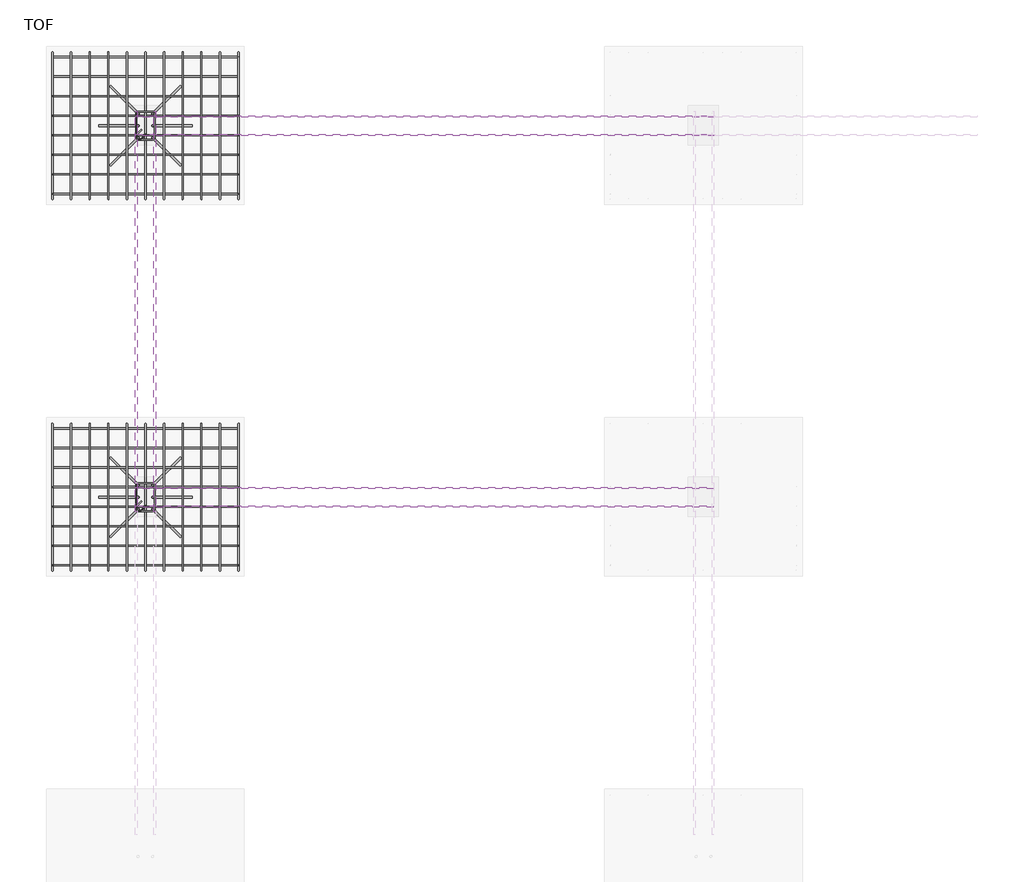
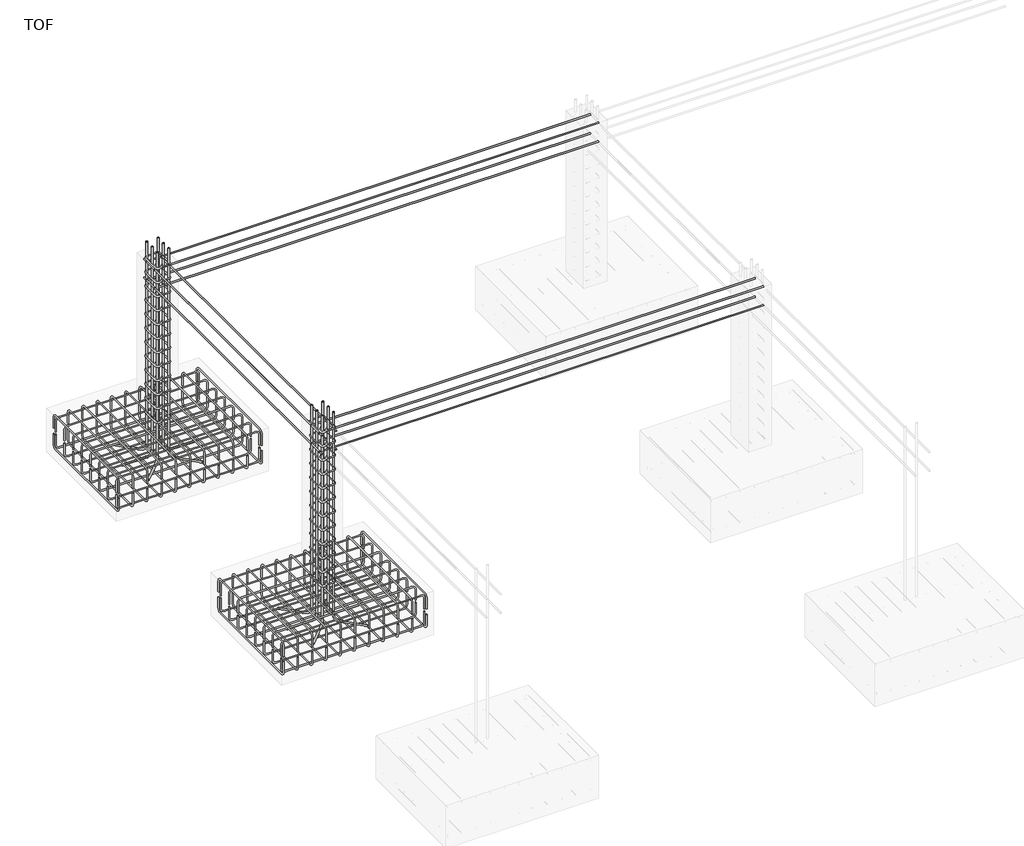
# One storey, part 3 of 10: 34 reinforcing bars.
"""IFC4 building model written with IfcOpenShell, lengths in millimetres."""

from ifc_helpers import new_model, si_unit, point, frame, origin, place, context, project, spatial, polyline, circle_curve, trimmed, segment, composite_curve, source, transform, mapped, element, save
from ifc_brep_helpers import swept_disk

model = new_model("IFC4")

# Units and contexts
model_context = context("Model", 3, world=origin())
ifc_project = project(units=[si_unit("LENGTHUNIT", "METRE", prefix="MILLI")], contexts=[model_context])

# Site, building, storey
site = spatial("IfcSite", under=ifc_project)
building = spatial("IfcBuilding", under=site)
storey = spatial("IfcBuildingStorey", under=building, Name="TOF", Elevation=-1828.8)

# Reinforcing bars
placement = place(None, origin())
reinforcing_bar_shape = source(origin(), model_context, "Body", "SolidModel", [
    swept_disk(composite_curve([segment(polyline([(-1914.7217857, -9959.6267376, -2018.8), (-1914.7217857, -9959.6267376, -1908.8)]), True, "CONTINUOUS"), segment(trimmed(circle_curve(frame((-1914.7217857, -9994.6267376, -1908.8), z_axis=(1.0, 0.0, 0.0), x_axis=(0.0, 35.0, 0.0)), 35.0), [point((-1914.7217857, -9959.6267376, -1908.8))], [point((-1914.7217857, -9994.6267376, -1873.8))], True, "CARTESIAN"), True, "CONTINUOUS"), segment(polyline([(-1914.7217857, -9994.6267376, -1873.8), (-1914.7217857, -11034.6267376, -1873.8)]), True, "CONTINUOUS"), segment(trimmed(circle_curve(frame((-1914.7217857, -11034.6267376, -1908.8), z_axis=(1.0, 0.0, 0.0), x_axis=(0.0, 0.0, 35.0)), 35.0), [point((-1914.7217857, -11034.6267376, -1873.8))], [point((-1914.7217857, -11069.6267376, -1908.8))], True, "CARTESIAN"), True, "CONTINUOUS"), segment(polyline([(-1914.7217857, -11069.6267376, -1908.8), (-1914.7217857, -11069.6267376, -2018.8)]), True, "CONTINUOUS")], self_intersect=False), 5.0),
])
element("IfcReinforcingBar", 1, at=placement, inside=storey, context=model_context, shape_type="MappedRepresentation", body=[
    mapped(reinforcing_bar_shape, transform((0.0, 0.0, 0.0), x_axis=(1.0, 0.0, 0.0), y_axis=(0.0, 1.0, 0.0), z_axis=(0.0, 0.0, 1.0))),
    mapped(reinforcing_bar_shape, transform((-141.0, 0.0, 0.0), x_axis=(1.0, 0.0, 0.0), y_axis=(0.0, 1.0, 0.0), z_axis=(0.0, 0.0, 1.0))),
    mapped(reinforcing_bar_shape, transform((-282.0, 0.0, 0.0), x_axis=(1.0, 0.0, 0.0), y_axis=(0.0, 1.0, 0.0), z_axis=(0.0, 0.0, 1.0))),
    mapped(reinforcing_bar_shape, transform((-423.0, 0.0, 0.0), x_axis=(1.0, 0.0, 0.0), y_axis=(0.0, 1.0, 0.0), z_axis=(0.0, 0.0, 1.0))),
    mapped(reinforcing_bar_shape, transform((-564.0, 0.0, 0.0), x_axis=(1.0, 0.0, 0.0), y_axis=(0.0, 1.0, 0.0), z_axis=(0.0, 0.0, 1.0))),
    mapped(reinforcing_bar_shape, transform((-705.0, 0.0, 0.0), x_axis=(1.0, 0.0, 0.0), y_axis=(0.0, 1.0, 0.0), z_axis=(0.0, 0.0, 1.0))),
    mapped(reinforcing_bar_shape, transform((-846.0, 0.0, 0.0), x_axis=(1.0, 0.0, 0.0), y_axis=(0.0, 1.0, 0.0), z_axis=(0.0, 0.0, 1.0))),
    mapped(reinforcing_bar_shape, transform((-987.0, 0.0, 0.0), x_axis=(1.0, 0.0, 0.0), y_axis=(0.0, 1.0, 0.0), z_axis=(0.0, 0.0, 1.0))),
    mapped(reinforcing_bar_shape, transform((-1128.0, 0.0, 0.0), x_axis=(1.0, 0.0, 0.0), y_axis=(0.0, 1.0, 0.0), z_axis=(0.0, 0.0, 1.0))),
    mapped(reinforcing_bar_shape, transform((-1269.0, 0.0, 0.0), x_axis=(1.0, 0.0, 0.0), y_axis=(0.0, 1.0, 0.0), z_axis=(0.0, 0.0, 1.0))),
    mapped(reinforcing_bar_shape, transform((-1410.0, 0.0, 0.0), x_axis=(1.0, 0.0, 0.0), y_axis=(0.0, 1.0, 0.0), z_axis=(0.0, 0.0, 1.0))),
])
reinforcing_bar_2_shape = source(origin(), model_context, "Body", "SolidModel", [
    swept_disk(composite_curve([segment(polyline([(-1914.7217857, -11069.6267376, -2077.5233378), (-1914.7217857, -11069.6267376, -2187.5233378)]), True, "CONTINUOUS"), segment(trimmed(circle_curve(frame((-1914.7217857, -11034.6267376, -2187.5233378), z_axis=(1.0, 0.0, 0.0), x_axis=(0.0, -35.0, 0.0)), 35.0), [point((-1914.7217857, -11069.6267376, -2187.5233378))], [point((-1914.7217857, -11034.6267376, -2222.5233378))], True, "CARTESIAN"), True, "CONTINUOUS"), segment(polyline([(-1914.7217857, -11034.6267376, -2222.5233378), (-1914.7217857, -9994.6267376, -2222.5233378)]), True, "CONTINUOUS"), segment(trimmed(circle_curve(frame((-1914.7217857, -9994.6267376, -2187.5233378), z_axis=(1.0, 0.0, 0.0), x_axis=(0.0, 0.0, -35.0)), 35.0), [point((-1914.7217857, -9994.6267376, -2222.5233378))], [point((-1914.7217857, -9959.6267376, -2187.5233378))], True, "CARTESIAN"), True, "CONTINUOUS"), segment(polyline([(-1914.7217857, -9959.6267376, -2187.5233378), (-1914.7217857, -9959.6267376, -2077.5233378)]), True, "CONTINUOUS")], self_intersect=False), 5.0),
])
element("IfcReinforcingBar", 2, at=placement, inside=storey, context=model_context, shape_type="MappedRepresentation", body=[
    mapped(reinforcing_bar_2_shape, transform((0.0, 0.0, 0.0), x_axis=(1.0, 0.0, 0.0), y_axis=(0.0, 1.0, 0.0), z_axis=(0.0, 0.0, 1.0))),
    mapped(reinforcing_bar_2_shape, transform((-141.0, 0.0, 0.0), x_axis=(1.0, 0.0, 0.0), y_axis=(0.0, 1.0, 0.0), z_axis=(0.0, 0.0, 1.0))),
    mapped(reinforcing_bar_2_shape, transform((-282.0, 0.0, 0.0), x_axis=(1.0, 0.0, 0.0), y_axis=(0.0, 1.0, 0.0), z_axis=(0.0, 0.0, 1.0))),
    mapped(reinforcing_bar_2_shape, transform((-423.0, 0.0, 0.0), x_axis=(1.0, 0.0, 0.0), y_axis=(0.0, 1.0, 0.0), z_axis=(0.0, 0.0, 1.0))),
    mapped(reinforcing_bar_2_shape, transform((-564.0, 0.0, 0.0), x_axis=(1.0, 0.0, 0.0), y_axis=(0.0, 1.0, 0.0), z_axis=(0.0, 0.0, 1.0))),
    mapped(reinforcing_bar_2_shape, transform((-705.0, 0.0, 0.0), x_axis=(1.0, 0.0, 0.0), y_axis=(0.0, 1.0, 0.0), z_axis=(0.0, 0.0, 1.0))),
    mapped(reinforcing_bar_2_shape, transform((-846.0, 0.0, 0.0), x_axis=(1.0, 0.0, 0.0), y_axis=(0.0, 1.0, 0.0), z_axis=(0.0, 0.0, 1.0))),
    mapped(reinforcing_bar_2_shape, transform((-987.0, 0.0, 0.0), x_axis=(1.0, 0.0, 0.0), y_axis=(0.0, 1.0, 0.0), z_axis=(0.0, 0.0, 1.0))),
    mapped(reinforcing_bar_2_shape, transform((-1128.0, 0.0, 0.0), x_axis=(1.0, 0.0, 0.0), y_axis=(0.0, 1.0, 0.0), z_axis=(0.0, 0.0, 1.0))),
    mapped(reinforcing_bar_2_shape, transform((-1269.0, 0.0, 0.0), x_axis=(1.0, 0.0, 0.0), y_axis=(0.0, 1.0, 0.0), z_axis=(0.0, 0.0, 1.0))),
    mapped(reinforcing_bar_2_shape, transform((-1410.0, 0.0, 0.0), x_axis=(1.0, 0.0, 0.0), y_axis=(0.0, 1.0, 0.0), z_axis=(0.0, 0.0, 1.0))),
])
reinforcing_bar_3_shape = source(origin(), model_context, "Body", "SolidModel", [
    swept_disk(composite_curve([segment(polyline([(-1914.7217857, -9994.6861459, -2066.1776706), (-1914.7217857, -9994.6861459, -2176.1776706)]), True, "CONTINUOUS"), segment(trimmed(circle_curve(frame((-1949.7217857, -9994.6861459, -2176.1776706), z_axis=(0.0, 1.0, 0.0), x_axis=(35.0, 0.0, 0.0)), 35.0), [point((-1914.7217857, -9994.6861459, -2176.1776706))], [point((-1949.7217857, -9994.6861459, -2211.1776706))], True, "CARTESIAN"), True, "CONTINUOUS"), segment(polyline([(-1949.7217857, -9994.6861459, -2211.1776706), (-3289.7217857, -9994.6861459, -2211.1776706)]), True, "CONTINUOUS"), segment(trimmed(circle_curve(frame((-3289.7217857, -9994.6861459, -2176.1776706), z_axis=(0.0, 1.0, 0.0), x_axis=(0.0, 0.0, -35.0)), 35.0), [point((-3289.7217857, -9994.6861459, -2211.1776706))], [point((-3324.7217857, -9994.6861459, -2176.1776706))], True, "CARTESIAN"), True, "CONTINUOUS"), segment(polyline([(-3324.7217857, -9994.6861459, -2176.1776706), (-3324.7217857, -9994.6861459, -2066.1776706)]), True, "CONTINUOUS")], self_intersect=False), 5.0),
])
element("IfcReinforcingBar", 3, at=placement, inside=storey, context=model_context, shape_type="MappedRepresentation", body=[
    mapped(reinforcing_bar_3_shape, transform((0.0, 0.0, 0.0), x_axis=(1.0, 0.0, 0.0), y_axis=(0.0, 1.0, 0.0), z_axis=(0.0, 0.0, 1.0))),
    mapped(reinforcing_bar_3_shape, transform((0.0, -148.0321606, 0.0), x_axis=(1.0, 0.0, 0.0), y_axis=(0.0, 1.0, 0.0), z_axis=(0.0, 0.0, 1.0))),
    mapped(reinforcing_bar_3_shape, transform((0.0, -296.0643211, 0.0), x_axis=(1.0, 0.0, 0.0), y_axis=(0.0, 1.0, 0.0), z_axis=(0.0, 0.0, 1.0))),
    mapped(reinforcing_bar_3_shape, transform((0.0, -444.0964817, 0.0), x_axis=(1.0, 0.0, 0.0), y_axis=(0.0, 1.0, 0.0), z_axis=(0.0, 0.0, 1.0))),
    mapped(reinforcing_bar_3_shape, transform((0.0, -592.1286423, 0.0), x_axis=(1.0, 0.0, 0.0), y_axis=(0.0, 1.0, 0.0), z_axis=(0.0, 0.0, 1.0))),
    mapped(reinforcing_bar_3_shape, transform((0.0, -740.1608029, 0.0), x_axis=(1.0, 0.0, 0.0), y_axis=(0.0, 1.0, 0.0), z_axis=(0.0, 0.0, 1.0))),
    mapped(reinforcing_bar_3_shape, transform((0.0, -888.1929634, 0.0), x_axis=(1.0, 0.0, 0.0), y_axis=(0.0, 1.0, 0.0), z_axis=(0.0, 0.0, 1.0))),
    mapped(reinforcing_bar_3_shape, transform((0.0, -1036.225124, 0.0), x_axis=(1.0, 0.0, 0.0), y_axis=(0.0, 1.0, 0.0), z_axis=(0.0, 0.0, 1.0))),
])
reinforcing_bar_4_shape = source(origin(), model_context, "Body", "SolidModel", [
    swept_disk(composite_curve([segment(polyline([(-1914.7217857, -11030.9112699, -2039.256778), (-1914.7217857, -11030.9112699, -1929.256778)]), True, "CONTINUOUS"), segment(trimmed(circle_curve(frame((-1949.7217857, -11030.9112699, -1929.256778), z_axis=(0.0, -1.0, 0.0), x_axis=(35.0, 0.0, 0.0)), 35.0), [point((-1914.7217857, -11030.9112699, -1929.256778))], [point((-1949.7217857, -11030.9112699, -1894.256778))], True, "CARTESIAN"), True, "CONTINUOUS"), segment(polyline([(-1949.7217857, -11030.9112699, -1894.256778), (-3289.7217857, -11030.9112699, -1894.256778)]), True, "CONTINUOUS"), segment(trimmed(circle_curve(frame((-3289.7217857, -11030.9112699, -1929.256778), z_axis=(0.0, -1.0, 0.0), x_axis=(0.0, 0.0, 35.0)), 35.0), [point((-3289.7217857, -11030.9112699, -1894.256778))], [point((-3324.7217857, -11030.9112699, -1929.256778))], True, "CARTESIAN"), True, "CONTINUOUS"), segment(polyline([(-3324.7217857, -11030.9112699, -1929.256778), (-3324.7217857, -11030.9112699, -2039.256778)]), True, "CONTINUOUS")], self_intersect=False), 5.0),
])
element("IfcReinforcingBar", 4, at=placement, inside=storey, context=model_context, shape_type="MappedRepresentation", body=[
    mapped(reinforcing_bar_4_shape, transform((0.0, 0.0, 0.0), x_axis=(1.0, 0.0, 0.0), y_axis=(0.0, 1.0, 0.0), z_axis=(0.0, 0.0, 1.0))),
    mapped(reinforcing_bar_4_shape, transform((0.0, 148.0321606, 0.0), x_axis=(1.0, 0.0, 0.0), y_axis=(0.0, 1.0, 0.0), z_axis=(0.0, 0.0, 1.0))),
    mapped(reinforcing_bar_4_shape, transform((0.0, 296.0643211, 0.0), x_axis=(1.0, 0.0, 0.0), y_axis=(0.0, 1.0, 0.0), z_axis=(0.0, 0.0, 1.0))),
    mapped(reinforcing_bar_4_shape, transform((0.0, 444.0964817, 0.0), x_axis=(1.0, 0.0, 0.0), y_axis=(0.0, 1.0, 0.0), z_axis=(0.0, 0.0, 1.0))),
    mapped(reinforcing_bar_4_shape, transform((0.0, 592.1286423, 0.0), x_axis=(1.0, 0.0, 0.0), y_axis=(0.0, 1.0, 0.0), z_axis=(0.0, 0.0, 1.0))),
    mapped(reinforcing_bar_4_shape, transform((0.0, 740.1608029, 0.0), x_axis=(1.0, 0.0, 0.0), y_axis=(0.0, 1.0, 0.0), z_axis=(0.0, 0.0, 1.0))),
    mapped(reinforcing_bar_4_shape, transform((0.0, 888.1929634, 0.0), x_axis=(1.0, 0.0, 0.0), y_axis=(0.0, 1.0, 0.0), z_axis=(0.0, 0.0, 1.0))),
    mapped(reinforcing_bar_4_shape, transform((0.0, 1036.225124, 0.0), x_axis=(1.0, 0.0, 0.0), y_axis=(0.0, 1.0, 0.0), z_axis=(0.0, 0.0, 1.0))),
])
reinforcing_bar_5_shape = source(origin(), model_context, "Body", "SolidModel", [
    swept_disk(composite_curve([segment(polyline([(-1914.7217857, -7144.6267376, -2018.8), (-1914.7217857, -7144.6267376, -1908.8)]), True, "CONTINUOUS"), segment(trimmed(circle_curve(frame((-1914.7217857, -7179.6267376, -1908.8), z_axis=(1.0, 0.0, 0.0), x_axis=(0.0, 35.0, 0.0)), 35.0), [point((-1914.7217857, -7144.6267376, -1908.8))], [point((-1914.7217857, -7179.6267376, -1873.8))], True, "CARTESIAN"), True, "CONTINUOUS"), segment(polyline([(-1914.7217857, -7179.6267376, -1873.8), (-1914.7217857, -8219.6267376, -1873.8)]), True, "CONTINUOUS"), segment(trimmed(circle_curve(frame((-1914.7217857, -8219.6267376, -1908.8), z_axis=(1.0, 0.0, 0.0), x_axis=(0.0, 0.0, 35.0)), 35.0), [point((-1914.7217857, -8219.6267376, -1873.8))], [point((-1914.7217857, -8254.6267376, -1908.8))], True, "CARTESIAN"), True, "CONTINUOUS"), segment(polyline([(-1914.7217857, -8254.6267376, -1908.8), (-1914.7217857, -8254.6267376, -2018.8)]), True, "CONTINUOUS")], self_intersect=False), 5.0),
])
element("IfcReinforcingBar", 5, at=placement, inside=storey, context=model_context, shape_type="MappedRepresentation", body=[
    mapped(reinforcing_bar_5_shape, transform((0.0, 0.0, 0.0), x_axis=(1.0, 0.0, 0.0), y_axis=(0.0, 1.0, 0.0), z_axis=(0.0, 0.0, 1.0))),
    mapped(reinforcing_bar_5_shape, transform((-141.0, 0.0, 0.0), x_axis=(1.0, 0.0, 0.0), y_axis=(0.0, 1.0, 0.0), z_axis=(0.0, 0.0, 1.0))),
    mapped(reinforcing_bar_5_shape, transform((-282.0, 0.0, 0.0), x_axis=(1.0, 0.0, 0.0), y_axis=(0.0, 1.0, 0.0), z_axis=(0.0, 0.0, 1.0))),
    mapped(reinforcing_bar_5_shape, transform((-423.0, 0.0, 0.0), x_axis=(1.0, 0.0, 0.0), y_axis=(0.0, 1.0, 0.0), z_axis=(0.0, 0.0, 1.0))),
    mapped(reinforcing_bar_5_shape, transform((-564.0, 0.0, 0.0), x_axis=(1.0, 0.0, 0.0), y_axis=(0.0, 1.0, 0.0), z_axis=(0.0, 0.0, 1.0))),
    mapped(reinforcing_bar_5_shape, transform((-705.0, 0.0, 0.0), x_axis=(1.0, 0.0, 0.0), y_axis=(0.0, 1.0, 0.0), z_axis=(0.0, 0.0, 1.0))),
    mapped(reinforcing_bar_5_shape, transform((-846.0, 0.0, 0.0), x_axis=(1.0, 0.0, 0.0), y_axis=(0.0, 1.0, 0.0), z_axis=(0.0, 0.0, 1.0))),
    mapped(reinforcing_bar_5_shape, transform((-987.0, 0.0, 0.0), x_axis=(1.0, 0.0, 0.0), y_axis=(0.0, 1.0, 0.0), z_axis=(0.0, 0.0, 1.0))),
    mapped(reinforcing_bar_5_shape, transform((-1128.0, 0.0, 0.0), x_axis=(1.0, 0.0, 0.0), y_axis=(0.0, 1.0, 0.0), z_axis=(0.0, 0.0, 1.0))),
    mapped(reinforcing_bar_5_shape, transform((-1269.0, 0.0, 0.0), x_axis=(1.0, 0.0, 0.0), y_axis=(0.0, 1.0, 0.0), z_axis=(0.0, 0.0, 1.0))),
    mapped(reinforcing_bar_5_shape, transform((-1410.0, 0.0, 0.0), x_axis=(1.0, 0.0, 0.0), y_axis=(0.0, 1.0, 0.0), z_axis=(0.0, 0.0, 1.0))),
])
reinforcing_bar_6_shape = source(origin(), model_context, "Body", "SolidModel", [
    swept_disk(composite_curve([segment(polyline([(-1914.7217857, -8254.6267376, -2077.5233378), (-1914.7217857, -8254.6267376, -2187.5233378)]), True, "CONTINUOUS"), segment(trimmed(circle_curve(frame((-1914.7217857, -8219.6267376, -2187.5233378), z_axis=(1.0, 0.0, 0.0), x_axis=(0.0, -35.0, 0.0)), 35.0), [point((-1914.7217857, -8254.6267376, -2187.5233378))], [point((-1914.7217857, -8219.6267376, -2222.5233378))], True, "CARTESIAN"), True, "CONTINUOUS"), segment(polyline([(-1914.7217857, -8219.6267376, -2222.5233378), (-1914.7217857, -7179.6267376, -2222.5233378)]), True, "CONTINUOUS"), segment(trimmed(circle_curve(frame((-1914.7217857, -7179.6267376, -2187.5233378), z_axis=(1.0, 0.0, 0.0), x_axis=(0.0, 0.0, -35.0)), 35.0), [point((-1914.7217857, -7179.6267376, -2222.5233378))], [point((-1914.7217857, -7144.6267376, -2187.5233378))], True, "CARTESIAN"), True, "CONTINUOUS"), segment(polyline([(-1914.7217857, -7144.6267376, -2187.5233378), (-1914.7217857, -7144.6267376, -2077.5233378)]), True, "CONTINUOUS")], self_intersect=False), 5.0),
])
element("IfcReinforcingBar", 6, at=placement, inside=storey, context=model_context, shape_type="MappedRepresentation", body=[
    mapped(reinforcing_bar_6_shape, transform((0.0, 0.0, 0.0), x_axis=(1.0, 0.0, 0.0), y_axis=(0.0, 1.0, 0.0), z_axis=(0.0, 0.0, 1.0))),
    mapped(reinforcing_bar_6_shape, transform((-141.0, 0.0, 0.0), x_axis=(1.0, 0.0, 0.0), y_axis=(0.0, 1.0, 0.0), z_axis=(0.0, 0.0, 1.0))),
    mapped(reinforcing_bar_6_shape, transform((-282.0, 0.0, 0.0), x_axis=(1.0, 0.0, 0.0), y_axis=(0.0, 1.0, 0.0), z_axis=(0.0, 0.0, 1.0))),
    mapped(reinforcing_bar_6_shape, transform((-423.0, 0.0, 0.0), x_axis=(1.0, 0.0, 0.0), y_axis=(0.0, 1.0, 0.0), z_axis=(0.0, 0.0, 1.0))),
    mapped(reinforcing_bar_6_shape, transform((-564.0, 0.0, 0.0), x_axis=(1.0, 0.0, 0.0), y_axis=(0.0, 1.0, 0.0), z_axis=(0.0, 0.0, 1.0))),
    mapped(reinforcing_bar_6_shape, transform((-705.0, 0.0, 0.0), x_axis=(1.0, 0.0, 0.0), y_axis=(0.0, 1.0, 0.0), z_axis=(0.0, 0.0, 1.0))),
    mapped(reinforcing_bar_6_shape, transform((-846.0, 0.0, 0.0), x_axis=(1.0, 0.0, 0.0), y_axis=(0.0, 1.0, 0.0), z_axis=(0.0, 0.0, 1.0))),
    mapped(reinforcing_bar_6_shape, transform((-987.0, 0.0, 0.0), x_axis=(1.0, 0.0, 0.0), y_axis=(0.0, 1.0, 0.0), z_axis=(0.0, 0.0, 1.0))),
    mapped(reinforcing_bar_6_shape, transform((-1128.0, 0.0, 0.0), x_axis=(1.0, 0.0, 0.0), y_axis=(0.0, 1.0, 0.0), z_axis=(0.0, 0.0, 1.0))),
    mapped(reinforcing_bar_6_shape, transform((-1269.0, 0.0, 0.0), x_axis=(1.0, 0.0, 0.0), y_axis=(0.0, 1.0, 0.0), z_axis=(0.0, 0.0, 1.0))),
    mapped(reinforcing_bar_6_shape, transform((-1410.0, 0.0, 0.0), x_axis=(1.0, 0.0, 0.0), y_axis=(0.0, 1.0, 0.0), z_axis=(0.0, 0.0, 1.0))),
])
reinforcing_bar_7_shape = source(origin(), model_context, "Body", "SolidModel", [
    swept_disk(composite_curve([segment(polyline([(-1914.7217857, -7179.6861459, -2066.1776706), (-1914.7217857, -7179.6861459, -2176.1776706)]), True, "CONTINUOUS"), segment(trimmed(circle_curve(frame((-1949.7217857, -7179.6861459, -2176.1776706), z_axis=(0.0, 1.0, 0.0), x_axis=(35.0, 0.0, 0.0)), 35.0), [point((-1914.7217857, -7179.6861459, -2176.1776706))], [point((-1949.7217857, -7179.6861459, -2211.1776706))], True, "CARTESIAN"), True, "CONTINUOUS"), segment(polyline([(-1949.7217857, -7179.6861459, -2211.1776706), (-3289.7217857, -7179.6861459, -2211.1776706)]), True, "CONTINUOUS"), segment(trimmed(circle_curve(frame((-3289.7217857, -7179.6861459, -2176.1776706), z_axis=(0.0, 1.0, 0.0), x_axis=(0.0, 0.0, -35.0)), 35.0), [point((-3289.7217857, -7179.6861459, -2211.1776706))], [point((-3324.7217857, -7179.6861459, -2176.1776706))], True, "CARTESIAN"), True, "CONTINUOUS"), segment(polyline([(-3324.7217857, -7179.6861459, -2176.1776706), (-3324.7217857, -7179.6861459, -2066.1776706)]), True, "CONTINUOUS")], self_intersect=False), 5.0),
])
element("IfcReinforcingBar", 7, at=placement, inside=storey, context=model_context, shape_type="MappedRepresentation", body=[
    mapped(reinforcing_bar_7_shape, transform((0.0, 0.0, 0.0), x_axis=(1.0, 0.0, 0.0), y_axis=(0.0, 1.0, 0.0), z_axis=(0.0, 0.0, 1.0))),
    mapped(reinforcing_bar_7_shape, transform((0.0, -148.0321606, 0.0), x_axis=(1.0, 0.0, 0.0), y_axis=(0.0, 1.0, 0.0), z_axis=(0.0, 0.0, 1.0))),
    mapped(reinforcing_bar_7_shape, transform((0.0, -296.0643211, 0.0), x_axis=(1.0, 0.0, 0.0), y_axis=(0.0, 1.0, 0.0), z_axis=(0.0, 0.0, 1.0))),
    mapped(reinforcing_bar_7_shape, transform((0.0, -444.0964817, 0.0), x_axis=(1.0, 0.0, 0.0), y_axis=(0.0, 1.0, 0.0), z_axis=(0.0, 0.0, 1.0))),
    mapped(reinforcing_bar_7_shape, transform((0.0, -592.1286423, 0.0), x_axis=(1.0, 0.0, 0.0), y_axis=(0.0, 1.0, 0.0), z_axis=(0.0, 0.0, 1.0))),
    mapped(reinforcing_bar_7_shape, transform((0.0, -740.1608029, 0.0), x_axis=(1.0, 0.0, 0.0), y_axis=(0.0, 1.0, 0.0), z_axis=(0.0, 0.0, 1.0))),
    mapped(reinforcing_bar_7_shape, transform((0.0, -888.1929634, 0.0), x_axis=(1.0, 0.0, 0.0), y_axis=(0.0, 1.0, 0.0), z_axis=(0.0, 0.0, 1.0))),
    mapped(reinforcing_bar_7_shape, transform((0.0, -1036.225124, 0.0), x_axis=(1.0, 0.0, 0.0), y_axis=(0.0, 1.0, 0.0), z_axis=(0.0, 0.0, 1.0))),
])
reinforcing_bar_8_shape = source(origin(), model_context, "Body", "SolidModel", [
    swept_disk(composite_curve([segment(polyline([(-1914.7217857, -8215.9112699, -2039.256778), (-1914.7217857, -8215.9112699, -1929.256778)]), True, "CONTINUOUS"), segment(trimmed(circle_curve(frame((-1949.7217857, -8215.9112699, -1929.256778), z_axis=(0.0, -1.0, 0.0), x_axis=(35.0, 0.0, 0.0)), 35.0), [point((-1914.7217857, -8215.9112699, -1929.256778))], [point((-1949.7217857, -8215.9112699, -1894.256778))], True, "CARTESIAN"), True, "CONTINUOUS"), segment(polyline([(-1949.7217857, -8215.9112699, -1894.256778), (-3289.7217857, -8215.9112699, -1894.256778)]), True, "CONTINUOUS"), segment(trimmed(circle_curve(frame((-3289.7217857, -8215.9112699, -1929.256778), z_axis=(0.0, -1.0, 0.0), x_axis=(0.0, 0.0, 35.0)), 35.0), [point((-3289.7217857, -8215.9112699, -1894.256778))], [point((-3324.7217857, -8215.9112699, -1929.256778))], True, "CARTESIAN"), True, "CONTINUOUS"), segment(polyline([(-3324.7217857, -8215.9112699, -1929.256778), (-3324.7217857, -8215.9112699, -2039.256778)]), True, "CONTINUOUS")], self_intersect=False), 5.0),
])
element("IfcReinforcingBar", 8, at=placement, inside=storey, context=model_context, shape_type="MappedRepresentation", body=[
    mapped(reinforcing_bar_8_shape, transform((0.0, 0.0, 0.0), x_axis=(1.0, 0.0, 0.0), y_axis=(0.0, 1.0, 0.0), z_axis=(0.0, 0.0, 1.0))),
    mapped(reinforcing_bar_8_shape, transform((0.0, 148.0321606, 0.0), x_axis=(1.0, 0.0, 0.0), y_axis=(0.0, 1.0, 0.0), z_axis=(0.0, 0.0, 1.0))),
    mapped(reinforcing_bar_8_shape, transform((0.0, 296.0643211, 0.0), x_axis=(1.0, 0.0, 0.0), y_axis=(0.0, 1.0, 0.0), z_axis=(0.0, 0.0, 1.0))),
    mapped(reinforcing_bar_8_shape, transform((0.0, 444.0964817, 0.0), x_axis=(1.0, 0.0, 0.0), y_axis=(0.0, 1.0, 0.0), z_axis=(0.0, 0.0, 1.0))),
    mapped(reinforcing_bar_8_shape, transform((0.0, 592.1286423, 0.0), x_axis=(1.0, 0.0, 0.0), y_axis=(0.0, 1.0, 0.0), z_axis=(0.0, 0.0, 1.0))),
    mapped(reinforcing_bar_8_shape, transform((0.0, 740.1608029, 0.0), x_axis=(1.0, 0.0, 0.0), y_axis=(0.0, 1.0, 0.0), z_axis=(0.0, 0.0, 1.0))),
    mapped(reinforcing_bar_8_shape, transform((0.0, 888.1929634, 0.0), x_axis=(1.0, 0.0, 0.0), y_axis=(0.0, 1.0, 0.0), z_axis=(0.0, 0.0, 1.0))),
    mapped(reinforcing_bar_8_shape, transform((0.0, 1036.225124, 0.0), x_axis=(1.0, 0.0, 0.0), y_axis=(0.0, 1.0, 0.0), z_axis=(0.0, 0.0, 1.0))),
])
reinforcing_bar_9_shape = source(origin(), model_context, "Body", "SolidModel", [
    swept_disk(composite_curve([segment(polyline([(-2649.751223, -10545.7150493, -1784.8), (-2683.6923485, -10579.6561748, -1784.8)]), True, "CONTINUOUS"), segment(trimmed(circle_curve(frame((-2666.7217857, -10596.6267376, -1784.8), z_axis=(0.0, 0.0, 1.0), x_axis=(-16.970562800000152, 16.970562799999243, 0.0)), 24.0), [point((-2683.6923485, -10579.6561748, -1784.8))], [point((-2666.7217857, -10620.6267376, -1784.8))], True, "CARTESIAN"), True, "CONTINUOUS"), segment(polyline([(-2666.7217857, -10620.6267376, -1784.8), (-2572.7217857, -10620.6267376, -1784.8)]), True, "CONTINUOUS"), segment(trimmed(circle_curve(frame((-2572.7217857, -10596.6267376, -1784.8), z_axis=(0.0, 0.0, 1.0), x_axis=(0.0, -24.0, 0.0)), 24.0), [point((-2572.7217857, -10620.6267376, -1784.8))], [point((-2548.7217857, -10596.6267376, -1784.8))], True, "CARTESIAN"), True, "CONTINUOUS"), segment(polyline([(-2548.7217857, -10596.6267376, -1784.8), (-2548.7217857, -10432.6267376, -1784.8)]), True, "CONTINUOUS"), segment(trimmed(circle_curve(frame((-2572.6837885, -10432.6267376, -1786.149972), z_axis=(-0.05624883273897078, 0.0, 0.9984167811167355), x_axis=(23.962002799999937, 0.0, 1.3499719999999797)), 24.0), [point((-2548.7217857, -10432.6267376, -1784.8))], [point((-2572.6837885, -10408.6267376, -1786.149972))], True, "CARTESIAN"), True, "CONTINUOUS"), segment(polyline([(-2572.6837885, -10408.6267376, -1786.149972), (-2666.759783, -10408.6267376, -1791.450028)]), True, "CONTINUOUS"), segment(trimmed(circle_curve(frame((-2666.759783, -10432.6267376, -1791.450028), z_axis=(-0.05624883273897078, 0.0, 0.9984167811167355), x_axis=(0.0, 24.0, 0.0)), 24.0), [point((-2666.759783, -10408.6267376, -1791.450028))], [point((-2690.7217857, -10432.6267376, -1792.8))], True, "CARTESIAN"), True, "CONTINUOUS"), segment(polyline([(-2690.7217857, -10432.6267376, -1792.8), (-2690.7217857, -10596.6267376, -1792.8)]), True, "CONTINUOUS"), segment(trimmed(circle_curve(frame((-2666.7217857, -10596.6267376, -1792.8), z_axis=(0.0, 0.0, 1.0), x_axis=(-24.0, 0.0, 0.0)), 24.0), [point((-2690.7217857, -10596.6267376, -1792.8))], [point((-2649.751223, -10613.5973003, -1792.8))], True, "CARTESIAN"), True, "CONTINUOUS"), segment(polyline([(-2649.751223, -10613.5973003, -1792.8), (-2615.8100975, -10579.6561748, -1792.8)]), True, "CONTINUOUS")], self_intersect=False), 4.0),
])
element("IfcReinforcingBar", 9, at=placement, inside=storey, context=model_context, shape_type="MappedRepresentation", body=[
    mapped(reinforcing_bar_9_shape, transform((0.0, 0.0, 0.0), x_axis=(1.0, 0.0, 0.0), y_axis=(0.0, 1.0, 0.0), z_axis=(0.0, 0.0, 1.0))),
    mapped(reinforcing_bar_9_shape, transform((0.0, 0.0, 145.9395608), x_axis=(1.0, 0.0, 0.0), y_axis=(0.0, 1.0, 0.0), z_axis=(0.0, 0.0, 1.0))),
    mapped(reinforcing_bar_9_shape, transform((0.0, 0.0, 291.8791216), x_axis=(1.0, 0.0, 0.0), y_axis=(0.0, 1.0, 0.0), z_axis=(0.0, 0.0, 1.0))),
    mapped(reinforcing_bar_9_shape, transform((0.0, 0.0, 437.8186825), x_axis=(1.0, 0.0, 0.0), y_axis=(0.0, 1.0, 0.0), z_axis=(0.0, 0.0, 1.0))),
    mapped(reinforcing_bar_9_shape, transform((0.0, 0.0, 583.7582433), x_axis=(1.0, 0.0, 0.0), y_axis=(0.0, 1.0, 0.0), z_axis=(0.0, 0.0, 1.0))),
    mapped(reinforcing_bar_9_shape, transform((0.0, 0.0, 729.6978041), x_axis=(1.0, 0.0, 0.0), y_axis=(0.0, 1.0, 0.0), z_axis=(0.0, 0.0, 1.0))),
    mapped(reinforcing_bar_9_shape, transform((0.0, 0.0, 875.6373649), x_axis=(1.0, 0.0, 0.0), y_axis=(0.0, 1.0, 0.0), z_axis=(0.0, 0.0, 1.0))),
    mapped(reinforcing_bar_9_shape, transform((0.0, 0.0, 1021.5769258), x_axis=(1.0, 0.0, 0.0), y_axis=(0.0, 1.0, 0.0), z_axis=(0.0, 0.0, 1.0))),
    mapped(reinforcing_bar_9_shape, transform((0.0, 0.0, 1167.5164866), x_axis=(1.0, 0.0, 0.0), y_axis=(0.0, 1.0, 0.0), z_axis=(0.0, 0.0, 1.0))),
    mapped(reinforcing_bar_9_shape, transform((0.0, 0.0, 1313.4560474), x_axis=(1.0, 0.0, 0.0), y_axis=(0.0, 1.0, 0.0), z_axis=(0.0, 0.0, 1.0))),
    mapped(reinforcing_bar_9_shape, transform((0.0, 0.0, 1459.3956082), x_axis=(1.0, 0.0, 0.0), y_axis=(0.0, 1.0, 0.0), z_axis=(0.0, 0.0, 1.0))),
    mapped(reinforcing_bar_9_shape, transform((0.0, 0.0, 1605.3351691), x_axis=(1.0, 0.0, 0.0), y_axis=(0.0, 1.0, 0.0), z_axis=(0.0, 0.0, 1.0))),
])
element("IfcReinforcingBar", 10, at=placement, inside=storey, context=model_context, shape_type="SolidModel", body=[
    swept_disk(composite_curve([segment(polyline([(-2564.115184, -10605.2333393, -20.0), (-2564.115184, -10605.2333393, -2138.7824747)]), True, "CONTINUOUS"), segment(trimmed(circle_curve(frame((-2524.8707576, -10644.4777657, -2138.7824747), z_axis=(-0.7071067811865545, -0.7071067811865406, 0.0), x_axis=(-39.244426400000066, 39.2444263999987, 0.0)), 55.5), [point((-2564.115184, -10605.2333393, -2138.7824747))], [point((-2524.8707576, -10644.4777657, -2194.2824747))], True, "CARTESIAN"), True, "CONTINUOUS"), segment(polyline([(-2524.8707576, -10644.4777657, -2194.2824747), (-2352.4916085, -10816.8569148, -2194.2824747)]), True, "CONTINUOUS")], self_intersect=False), 8.0),
])
element("IfcReinforcingBar", 11, at=placement, inside=storey, context=model_context, shape_type="SolidModel", body=[
    swept_disk(composite_curve([segment(polyline([(-2564.065184, -10514.6267376, -20.0), (-2564.065184, -10514.6267376, -2138.7824747)]), True, "CONTINUOUS"), segment(trimmed(circle_curve(frame((-2508.565184, -10514.6267376, -2138.7824747), z_axis=(0.0, -1.0, 0.0), x_axis=(-55.5, 0.0, 0.0)), 55.5), [point((-2564.065184, -10514.6267376, -2138.7824747))], [point((-2508.565184, -10514.6267376, -2194.2824747))], True, "CARTESIAN"), True, "CONTINUOUS"), segment(polyline([(-2508.565184, -10514.6267376, -2194.2824747), (-2264.8342534, -10514.6267376, -2194.2824747)]), True, "CONTINUOUS")], self_intersect=False), 8.0),
])
element("IfcReinforcingBar", 12, at=placement, inside=storey, context=model_context, shape_type="SolidModel", body=[
    swept_disk(composite_curve([segment(polyline([(-2564.115184, -10424.0201359, -20.0), (-2564.115184, -10424.0201359, -2138.7824747)]), True, "CONTINUOUS"), segment(trimmed(circle_curve(frame((-2524.8707576, -10384.7757095, -2138.7824747), z_axis=(0.7071067811865545, -0.7071067811865407, 0.0), x_axis=(-39.244426400000066, -39.24442640000052, 0.0)), 55.5), [point((-2564.115184, -10424.0201359, -2138.7824747))], [point((-2524.8707576, -10384.7757095, -2194.2824747))], True, "CARTESIAN"), True, "CONTINUOUS"), segment(polyline([(-2524.8707576, -10384.7757095, -2194.2824747), (-2352.4916085, -10212.3965603, -2194.2824747)]), True, "CONTINUOUS")], self_intersect=False), 8.0),
])
element("IfcReinforcingBar", 13, at=placement, inside=storey, context=model_context, shape_type="SolidModel", body=[
    swept_disk(composite_curve([segment(polyline([(-2675.3283874, -10605.2333393, -20.0), (-2675.3283874, -10605.2333393, -2138.7824747)]), True, "CONTINUOUS"), segment(trimmed(circle_curve(frame((-2714.5728138, -10644.4777657, -2138.7824747), z_axis=(-0.7071067811865517, 0.7071067811865434, 0.0), x_axis=(39.244426400000066, 39.2444263999987, 0.0)), 55.5), [point((-2675.3283874, -10605.2333393, -2138.7824747))], [point((-2714.5728138, -10644.4777657, -2194.2824747))], True, "CARTESIAN"), True, "CONTINUOUS"), segment(polyline([(-2714.5728138, -10644.4777657, -2194.2824747), (-2886.951963, -10816.8569148, -2194.2824747)]), True, "CONTINUOUS")], self_intersect=False), 8.0),
])
element("IfcReinforcingBar", 14, at=placement, inside=storey, context=model_context, shape_type="SolidModel", body=[
    swept_disk(composite_curve([segment(polyline([(-2675.3783874, -10514.6267376, -20.0), (-2675.3783874, -10514.6267376, -2138.7824747)]), True, "CONTINUOUS"), segment(trimmed(circle_curve(frame((-2730.8783874, -10514.6267376, -2138.7824747), z_axis=(0.0, 1.0, 0.0), x_axis=(55.5, 0.0, 0.0)), 55.5), [point((-2675.3783874, -10514.6267376, -2138.7824747))], [point((-2730.8783874, -10514.6267376, -2194.2824747))], True, "CARTESIAN"), True, "CONTINUOUS"), segment(polyline([(-2730.8783874, -10514.6267376, -2194.2824747), (-2974.6093181, -10514.6267376, -2194.2824747)]), True, "CONTINUOUS")], self_intersect=False), 8.0),
])
element("IfcReinforcingBar", 15, at=placement, inside=storey, context=model_context, shape_type="SolidModel", body=[
    swept_disk(composite_curve([segment(polyline([(-2675.3283874, -10424.0201359, -20.0), (-2675.3283874, -10424.0201359, -2138.7824747)]), True, "CONTINUOUS"), segment(trimmed(circle_curve(frame((-2714.5728138, -10384.7757095, -2138.7824747), z_axis=(0.7071067811865572, 0.7071067811865379, 0.0), x_axis=(39.244426400000066, -39.24442640000052, 0.0)), 55.5), [point((-2675.3283874, -10424.0201359, -2138.7824747))], [point((-2714.5728138, -10384.7757095, -2194.2824747))], True, "CARTESIAN"), True, "CONTINUOUS"), segment(polyline([(-2714.5728138, -10384.7757095, -2194.2824747), (-2886.951963, -10212.3965603, -2194.2824747)]), True, "CONTINUOUS")], self_intersect=False), 8.0),
])
reinforcing_bar_10_shape = source(origin(), model_context, "Body", "SolidModel", [
    swept_disk(composite_curve([segment(polyline([(-2649.751223, -7730.7150493, -1784.8), (-2683.6923485, -7764.6561748, -1784.8)]), True, "CONTINUOUS"), segment(trimmed(circle_curve(frame((-2666.7217857, -7781.6267376, -1784.8), z_axis=(0.0, 0.0, 1.0), x_axis=(-16.970562800000152, 16.970562799999243, 0.0)), 24.0), [point((-2683.6923485, -7764.6561748, -1784.8))], [point((-2666.7217857, -7805.6267376, -1784.8))], True, "CARTESIAN"), True, "CONTINUOUS"), segment(polyline([(-2666.7217857, -7805.6267376, -1784.8), (-2572.7217857, -7805.6267376, -1784.8)]), True, "CONTINUOUS"), segment(trimmed(circle_curve(frame((-2572.7217857, -7781.6267376, -1784.8), z_axis=(0.0, 0.0, 1.0), x_axis=(0.0, -24.0, 0.0)), 24.0), [point((-2572.7217857, -7805.6267376, -1784.8))], [point((-2548.7217857, -7781.6267376, -1784.8))], True, "CARTESIAN"), True, "CONTINUOUS"), segment(polyline([(-2548.7217857, -7781.6267376, -1784.8), (-2548.7217857, -7617.6267376, -1784.8)]), True, "CONTINUOUS"), segment(trimmed(circle_curve(frame((-2572.6837885, -7617.6267376, -1786.149972), z_axis=(-0.05624883273897078, 0.0, 0.9984167811167355), x_axis=(23.962002799999937, 0.0, 1.3499719999999797)), 24.0), [point((-2548.7217857, -7617.6267376, -1784.8))], [point((-2572.6837885, -7593.6267376, -1786.149972))], True, "CARTESIAN"), True, "CONTINUOUS"), segment(polyline([(-2572.6837885, -7593.6267376, -1786.149972), (-2666.759783, -7593.6267376, -1791.450028)]), True, "CONTINUOUS"), segment(trimmed(circle_curve(frame((-2666.759783, -7617.6267376, -1791.450028), z_axis=(-0.05624883273897078, 0.0, 0.9984167811167355), x_axis=(0.0, 24.0, 0.0)), 24.0), [point((-2666.759783, -7593.6267376, -1791.450028))], [point((-2690.7217857, -7617.6267376, -1792.8))], True, "CARTESIAN"), True, "CONTINUOUS"), segment(polyline([(-2690.7217857, -7617.6267376, -1792.8), (-2690.7217857, -7781.6267376, -1792.8)]), True, "CONTINUOUS"), segment(trimmed(circle_curve(frame((-2666.7217857, -7781.6267376, -1792.8), z_axis=(0.0, 0.0, 1.0), x_axis=(-24.0, 0.0, 0.0)), 24.0), [point((-2690.7217857, -7781.6267376, -1792.8))], [point((-2649.751223, -7798.5973003, -1792.8))], True, "CARTESIAN"), True, "CONTINUOUS"), segment(polyline([(-2649.751223, -7798.5973003, -1792.8), (-2615.8100975, -7764.6561748, -1792.8)]), True, "CONTINUOUS")], self_intersect=False), 4.0),
])
element("IfcReinforcingBar", 16, at=placement, inside=storey, context=model_context, shape_type="MappedRepresentation", body=[
    mapped(reinforcing_bar_10_shape, transform((0.0, 0.0, 0.0), x_axis=(1.0, 0.0, 0.0), y_axis=(0.0, 1.0, 0.0), z_axis=(0.0, 0.0, 1.0))),
    mapped(reinforcing_bar_10_shape, transform((0.0, 0.0, 145.9395608), x_axis=(1.0, 0.0, 0.0), y_axis=(0.0, 1.0, 0.0), z_axis=(0.0, 0.0, 1.0))),
    mapped(reinforcing_bar_10_shape, transform((0.0, 0.0, 291.8791216), x_axis=(1.0, 0.0, 0.0), y_axis=(0.0, 1.0, 0.0), z_axis=(0.0, 0.0, 1.0))),
    mapped(reinforcing_bar_10_shape, transform((0.0, 0.0, 437.8186825), x_axis=(1.0, 0.0, 0.0), y_axis=(0.0, 1.0, 0.0), z_axis=(0.0, 0.0, 1.0))),
    mapped(reinforcing_bar_10_shape, transform((0.0, 0.0, 583.7582433), x_axis=(1.0, 0.0, 0.0), y_axis=(0.0, 1.0, 0.0), z_axis=(0.0, 0.0, 1.0))),
    mapped(reinforcing_bar_10_shape, transform((0.0, 0.0, 729.6978041), x_axis=(1.0, 0.0, 0.0), y_axis=(0.0, 1.0, 0.0), z_axis=(0.0, 0.0, 1.0))),
    mapped(reinforcing_bar_10_shape, transform((0.0, 0.0, 875.6373649), x_axis=(1.0, 0.0, 0.0), y_axis=(0.0, 1.0, 0.0), z_axis=(0.0, 0.0, 1.0))),
    mapped(reinforcing_bar_10_shape, transform((0.0, 0.0, 1021.5769258), x_axis=(1.0, 0.0, 0.0), y_axis=(0.0, 1.0, 0.0), z_axis=(0.0, 0.0, 1.0))),
    mapped(reinforcing_bar_10_shape, transform((0.0, 0.0, 1167.5164866), x_axis=(1.0, 0.0, 0.0), y_axis=(0.0, 1.0, 0.0), z_axis=(0.0, 0.0, 1.0))),
    mapped(reinforcing_bar_10_shape, transform((0.0, 0.0, 1313.4560474), x_axis=(1.0, 0.0, 0.0), y_axis=(0.0, 1.0, 0.0), z_axis=(0.0, 0.0, 1.0))),
    mapped(reinforcing_bar_10_shape, transform((0.0, 0.0, 1459.3956082), x_axis=(1.0, 0.0, 0.0), y_axis=(0.0, 1.0, 0.0), z_axis=(0.0, 0.0, 1.0))),
    mapped(reinforcing_bar_10_shape, transform((0.0, 0.0, 1605.3351691), x_axis=(1.0, 0.0, 0.0), y_axis=(0.0, 1.0, 0.0), z_axis=(0.0, 0.0, 1.0))),
])
element("IfcReinforcingBar", 17, at=placement, inside=storey, context=model_context, shape_type="SolidModel", body=[
    swept_disk(composite_curve([segment(polyline([(-2564.115184, -7790.2333393, -20.0), (-2564.115184, -7790.2333393, -2138.7824747)]), True, "CONTINUOUS"), segment(trimmed(circle_curve(frame((-2524.8707576, -7829.4777657, -2138.7824747), z_axis=(-0.7071067811865545, -0.7071067811865406, 0.0), x_axis=(-39.244426400000066, 39.24442640000052, 0.0)), 55.5), [point((-2564.115184, -7790.2333393, -2138.7824747))], [point((-2524.8707576, -7829.4777657, -2194.2824747))], True, "CARTESIAN"), True, "CONTINUOUS"), segment(polyline([(-2524.8707576, -7829.4777657, -2194.2824747), (-2352.4916085, -8001.8569148, -2194.2824747)]), True, "CONTINUOUS")], self_intersect=False), 8.0),
])
element("IfcReinforcingBar", 18, at=placement, inside=storey, context=model_context, shape_type="SolidModel", body=[
    swept_disk(composite_curve([segment(polyline([(-2564.065184, -7699.6267376, -20.0), (-2564.065184, -7699.6267376, -2138.7824747)]), True, "CONTINUOUS"), segment(trimmed(circle_curve(frame((-2508.565184, -7699.6267376, -2138.7824747), z_axis=(0.0, -1.0, 0.0), x_axis=(-55.5, 0.0, 0.0)), 55.5), [point((-2564.065184, -7699.6267376, -2138.7824747))], [point((-2508.565184, -7699.6267376, -2194.2824747))], True, "CARTESIAN"), True, "CONTINUOUS"), segment(polyline([(-2508.565184, -7699.6267376, -2194.2824747), (-2264.8342534, -7699.6267376, -2194.2824747)]), True, "CONTINUOUS")], self_intersect=False), 8.0),
])
element("IfcReinforcingBar", 19, at=placement, inside=storey, context=model_context, shape_type="SolidModel", body=[
    swept_disk(composite_curve([segment(polyline([(-2564.115184, -7609.0201359, -20.0), (-2564.115184, -7609.0201359, -2138.7824747)]), True, "CONTINUOUS"), segment(trimmed(circle_curve(frame((-2524.8707576, -7569.7757095, -2138.7824747), z_axis=(0.7071067811865545, -0.7071067811865407, 0.0), x_axis=(-39.244426400000066, -39.24442640000052, 0.0)), 55.5), [point((-2564.115184, -7609.0201359, -2138.7824747))], [point((-2524.8707576, -7569.7757095, -2194.2824747))], True, "CARTESIAN"), True, "CONTINUOUS"), segment(polyline([(-2524.8707576, -7569.7757095, -2194.2824747), (-2352.4916085, -7397.3965603, -2194.2824747)]), True, "CONTINUOUS")], self_intersect=False), 8.0),
])
element("IfcReinforcingBar", 20, at=placement, inside=storey, context=model_context, shape_type="SolidModel", body=[
    swept_disk(composite_curve([segment(polyline([(-2675.3283874, -7790.2333393, -20.0), (-2675.3283874, -7790.2333393, -2138.7824747)]), True, "CONTINUOUS"), segment(trimmed(circle_curve(frame((-2714.5728138, -7829.4777657, -2138.7824747), z_axis=(-0.7071067811865517, 0.7071067811865434, 0.0), x_axis=(39.244426400000066, 39.24442640000052, 0.0)), 55.5), [point((-2675.3283874, -7790.2333393, -2138.7824747))], [point((-2714.5728138, -7829.4777657, -2194.2824747))], True, "CARTESIAN"), True, "CONTINUOUS"), segment(polyline([(-2714.5728138, -7829.4777657, -2194.2824747), (-2886.951963, -8001.8569148, -2194.2824747)]), True, "CONTINUOUS")], self_intersect=False), 8.0),
])
element("IfcReinforcingBar", 21, at=placement, inside=storey, context=model_context, shape_type="SolidModel", body=[
    swept_disk(composite_curve([segment(polyline([(-2675.3783874, -7699.6267376, -20.0), (-2675.3783874, -7699.6267376, -2138.7824747)]), True, "CONTINUOUS"), segment(trimmed(circle_curve(frame((-2730.8783874, -7699.6267376, -2138.7824747), z_axis=(0.0, 1.0, 0.0), x_axis=(55.5, 0.0, 0.0)), 55.5), [point((-2675.3783874, -7699.6267376, -2138.7824747))], [point((-2730.8783874, -7699.6267376, -2194.2824747))], True, "CARTESIAN"), True, "CONTINUOUS"), segment(polyline([(-2730.8783874, -7699.6267376, -2194.2824747), (-2974.6093181, -7699.6267376, -2194.2824747)]), True, "CONTINUOUS")], self_intersect=False), 8.0),
])
element("IfcReinforcingBar", 22, at=placement, inside=storey, context=model_context, shape_type="SolidModel", body=[
    swept_disk(composite_curve([segment(polyline([(-2675.3283874, -7609.0201359, -20.0), (-2675.3283874, -7609.0201359, -2138.7824747)]), True, "CONTINUOUS"), segment(trimmed(circle_curve(frame((-2714.5728138, -7569.7757095, -2138.7824747), z_axis=(0.7071067811865572, 0.7071067811865379, 0.0), x_axis=(39.244426400000066, -39.24442640000052, 0.0)), 55.5), [point((-2675.3283874, -7609.0201359, -2138.7824747))], [point((-2714.5728138, -7569.7757095, -2194.2824747))], True, "CARTESIAN"), True, "CONTINUOUS"), segment(polyline([(-2714.5728138, -7569.7757095, -2194.2824747), (-2886.951963, -7397.3965603, -2194.2824747)]), True, "CONTINUOUS")], self_intersect=False), 8.0),
])
element("IfcReinforcingBar", 23, at=placement, inside=storey, context=model_context, shape_type="SolidModel", body=[
    swept_disk(composite_curve([segment(polyline([(1685.2782143, -10584.5917105, -210.0508449), (-2694.7217857, -10584.5917105, -210.0508449)]), True, "CONTINUOUS")], self_intersect=False), 6.0),
])
element("IfcReinforcingBar", 24, at=placement, inside=storey, context=model_context, shape_type="SolidModel", body=[
    swept_disk(composite_curve([segment(polyline([(1685.2782143, -10584.5917105, -405.0508449), (-2694.7217857, -10584.5917105, -405.0508449)]), True, "CONTINUOUS")], self_intersect=False), 6.0),
])
element("IfcReinforcingBar", 25, at=placement, inside=storey, context=model_context, shape_type="SolidModel", body=[
    swept_disk(composite_curve([segment(polyline([(1685.2782143, -10444.6617646, -210.0508449), (-2694.7217857, -10444.6617646, -210.0508449)]), True, "CONTINUOUS")], self_intersect=False), 6.0),
])
element("IfcReinforcingBar", 26, at=placement, inside=storey, context=model_context, shape_type="SolidModel", body=[
    swept_disk(composite_curve([segment(polyline([(1685.2782143, -10444.6617646, -405.0508449), (-2694.7217857, -10444.6617646, -405.0508449)]), True, "CONTINUOUS")], self_intersect=False), 6.0),
])
element("IfcReinforcingBar", 27, at=placement, inside=storey, context=model_context, shape_type="SolidModel", body=[
    swept_disk(composite_curve([segment(polyline([(1685.2782143, -7769.5917105, -210.0508449), (-2694.7217857, -7769.5917105, -210.0508449)]), True, "CONTINUOUS")], self_intersect=False), 6.0),
])
element("IfcReinforcingBar", 28, at=placement, inside=storey, context=model_context, shape_type="SolidModel", body=[
    swept_disk(composite_curve([segment(polyline([(1685.2782143, -7769.5917105, -405.0508449), (-2694.7217857, -7769.5917105, -405.0508449)]), True, "CONTINUOUS")], self_intersect=False), 6.0),
])
element("IfcReinforcingBar", 29, at=placement, inside=storey, context=model_context, shape_type="SolidModel", body=[
    swept_disk(composite_curve([segment(polyline([(1685.2782143, -7629.6617646, -210.0508449), (-2694.7217857, -7629.6617646, -210.0508449)]), True, "CONTINUOUS")], self_intersect=False), 6.0),
])
element("IfcReinforcingBar", 30, at=placement, inside=storey, context=model_context, shape_type="SolidModel", body=[
    swept_disk(composite_curve([segment(polyline([(1685.2782143, -7629.6617646, -405.0508449), (-2694.7217857, -7629.6617646, -405.0508449)]), True, "CONTINUOUS")], self_intersect=False), 6.0),
])
element("IfcReinforcingBar", 31, at=placement, inside=storey, context=model_context, shape_type="SolidModel", body=[
    swept_disk(composite_curve([segment(polyline([(-2689.6867587, -10624.6267376, -210.0508449), (-2689.6867587, -7589.6267376, -210.0508449)]), True, "CONTINUOUS")], self_intersect=False), 6.0),
])
element("IfcReinforcingBar", 32, at=placement, inside=storey, context=model_context, shape_type="SolidModel", body=[
    swept_disk(composite_curve([segment(polyline([(-2689.6867587, -10624.6267376, -405.0508449), (-2689.6867587, -7589.6267376, -405.0508449)]), True, "CONTINUOUS")], self_intersect=False), 6.0),
])
element("IfcReinforcingBar", 33, at=placement, inside=storey, context=model_context, shape_type="SolidModel", body=[
    swept_disk(composite_curve([segment(polyline([(-2549.7568128, -10624.6267376, -210.0508449), (-2549.7568128, -7589.6267376, -210.0508449)]), True, "CONTINUOUS")], self_intersect=False), 6.0),
])
element("IfcReinforcingBar", 34, at=placement, inside=storey, context=model_context, shape_type="SolidModel", body=[
    swept_disk(composite_curve([segment(polyline([(-2549.7568128, -10624.6267376, -405.0508449), (-2549.7568128, -7589.6267376, -405.0508449)]), True, "CONTINUOUS")], self_intersect=False), 6.0),
])

save(model, "model.ifc")

# Revit data of these elements
# Elements 1, 2, 3, 4, 5, 6, 7, 8, 9, 10, 11, 12, 13, 14, 15, 16, 17, 18, 19, 20, 21, 22, 23, 24, 25, 26, 27, 28, 29, 30, 31, 32, 33, 34 (IfcReinforcingBar)
#   Phase Created = New Construction
